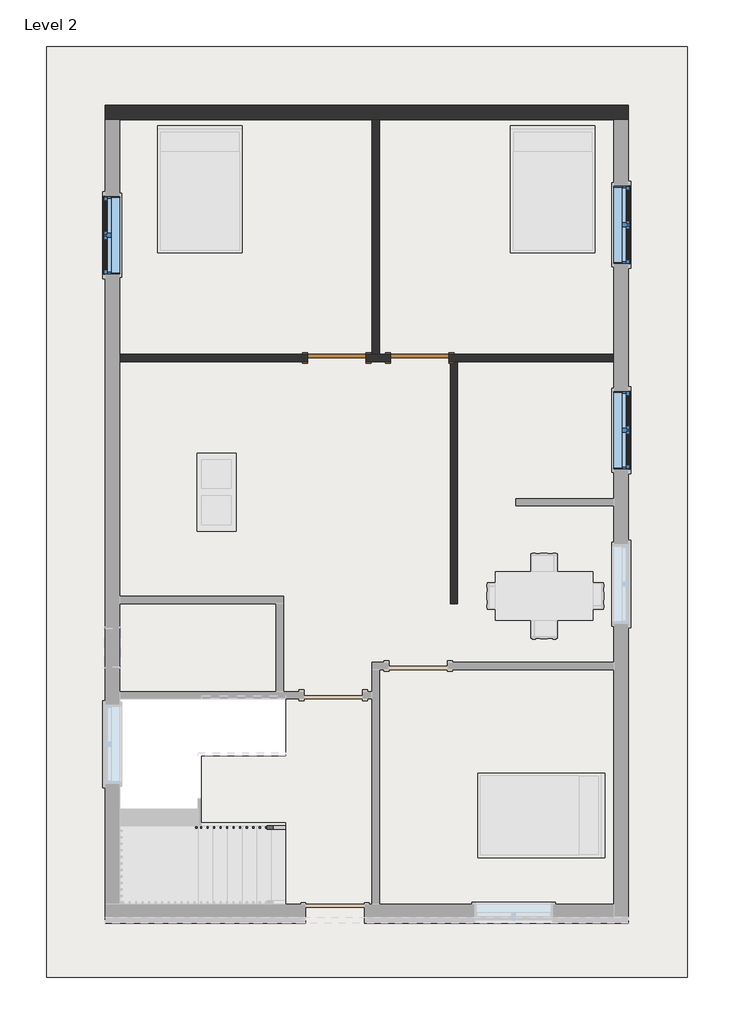
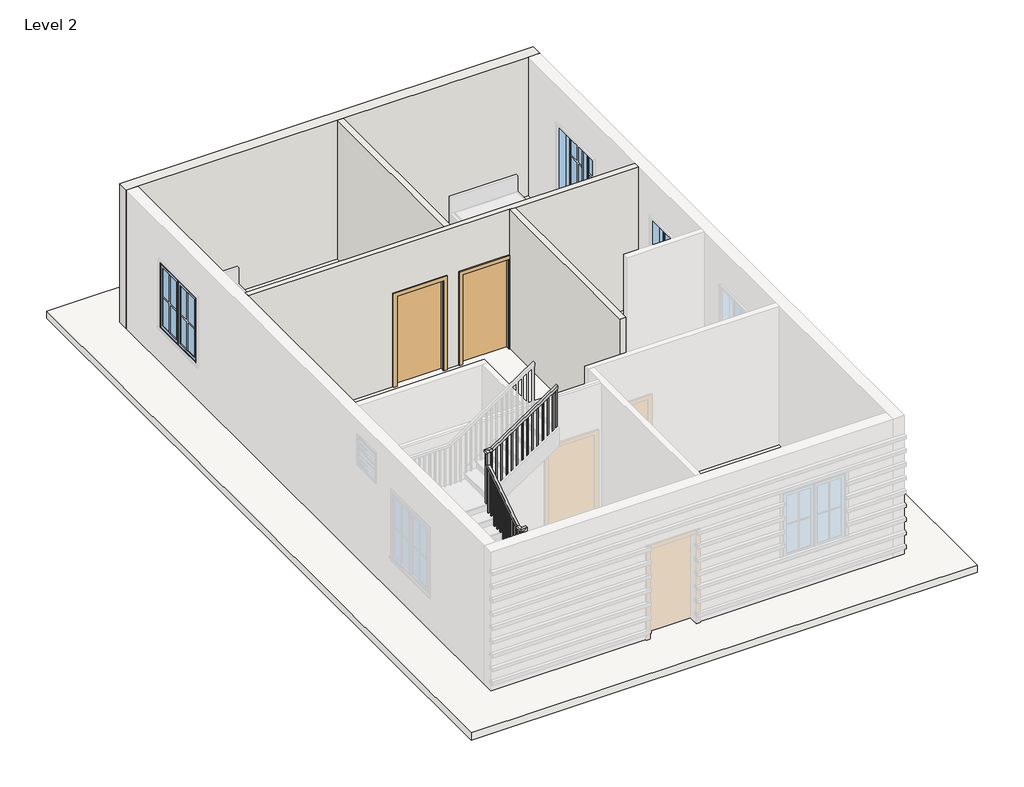
# One storey, part 2 of 3: 4 walls, 3 windows, 2 doors, 1 railing, 1 roof.
"""IFC4 building model written with IfcOpenShell, lengths in millimetres."""

from ifc_helpers import new_model, si_unit, frame, origin, place, context, project, spatial, polyline, outline, extrude, faceted_brep, transform, mapped, element, save
from components import single_flush_door_3_17d80c48, single_flush_door_3_5e62189b, window_casement_double_window_4_576b2d2c

model = new_model("IFC4")

# Units and contexts
model_context = context("Model", 3, world=origin())
ifc_project = project(units=[si_unit("LENGTHUNIT", "METRE", prefix="MILLI")], contexts=[model_context])

# Site, building, storey
site = spatial("IfcSite", under=ifc_project)
building = spatial("IfcBuilding", under=site)
storey = spatial("IfcBuildingStorey", under=building, Name="Level 2", Elevation=3048.0)

# Doors
placement = place(None, origin())
single_flush_door_3_shape = single_flush_door_3_17d80c48(model_context)
element("IfcDoor", 1, ObjectType="Single-Flush : DOOR 3'", at=placement, inside=storey, context=model_context, shape_type="MappedRepresentation", body=[
    mapped(single_flush_door_3_shape, transform((-1721.4617403, 2133.1073441, 3048.0), x_axis=(1.0, 0.0, 0.0), y_axis=(0.0, 1.0, 0.0), z_axis=(0.0, 0.0, 1.0))),
])
single_flush_door_3_2_shape = single_flush_door_3_5e62189b(model_context)
element("IfcDoor", 2, ObjectType="Single-Flush : DOOR 3'", at=placement, inside=storey, context=model_context, shape_type="MappedRepresentation", body=[
    mapped(single_flush_door_3_2_shape, transform((-426.0617403, 2133.1073441, 3048.0), x_axis=(-1.0, 0.0, 0.0), y_axis=(0.0, -1.0, 0.0), z_axis=(0.0, 0.0, 1.0))),
])

# Railing
element("IfcRailing", 3, ObjectType="Handrail - Rectangular", at=placement, inside=storey, context=model_context, shape_type="SolidModel", body=[
    faceted_brep([(-2515.2117403, -5213.8426559, 4114.8), (-2515.2117403, -5213.8426559, 4053.7459984), (-2515.2117403, -5163.0426559, 4053.7459984), (-2515.2117403, -5163.0426559, 4114.8), (-3810.6117403, -5213.8426559, 4978.4), (-3861.4117403, -5213.8426559, 4951.2126651), (-3861.4117403, -5163.0426559, 4951.2126651), (-3810.6117403, -5163.0426559, 4978.4), (-3810.6117403, -5213.8426559, 5232.4), (-3861.4117403, -5213.8426559, 5181.6), (-3861.4117403, -5163.0426559, 5181.6), (-3810.6117403, -5163.0426559, 5232.4), (-3937.6117403, -5213.8426559, 5232.4), (-3937.6117403, -5213.8426559, 5181.6), (-3886.8117403, -5163.0426559, 5181.6), (-3886.8117403, -5163.0426559, 5232.4), (-3937.6117403, -5086.8426559, 5232.4), (-3937.6117403, -5071.4616535, 5181.6), (-3886.8117403, -5071.4616535, 5181.6), (-3886.8117403, -5086.8426559, 5232.4), (-3937.6117403, -4096.2426559, 5892.8), (-3937.6117403, -4045.4426559, 5865.6126651), (-3886.8117403, -4045.4426559, 5865.6126651), (-3886.8117403, -4096.2426559, 5892.8), (-3937.6117403, -4096.2426559, 6146.8), (-3937.6117403, -4045.4426559, 6096.0), (-3886.8117403, -4045.4426559, 6096.0), (-3886.8117403, -4096.2426559, 6146.8), (-3937.6117403, -3969.2426559, 6146.8), (-3937.6117403, -3969.2426559, 6096.0), (-3886.8117403, -4020.0426559, 6096.0), (-3886.8117403, -4020.0426559, 6146.8), (-3810.6117403, -3969.2426559, 6146.8), (-3795.2307379, -3969.2426559, 6096.0), (-3795.2307379, -4020.0426559, 6096.0), (-3810.6117403, -4020.0426559, 6146.8), (-2515.2117403, -3969.2426559, 7010.4), (-2515.2117403, -4020.0426559, 7010.4), (-2515.2117403, -4020.0426559, 6949.3459984), (-2515.2117403, -3969.2426559, 6949.3459984)], [[[0, 1, 2, 3]], [[1, 0, 4, 5]], [[2, 1, 5, 6]], [[3, 2, 6, 7]], [[0, 3, 7, 4]], [[5, 4, 8, 9]], [[6, 5, 9, 10]], [[7, 6, 10, 11]], [[4, 7, 11, 8]], [[9, 8, 12, 13]], [[10, 9, 13, 14]], [[11, 10, 14, 15]], [[8, 11, 15, 12]], [[13, 12, 16, 17]], [[14, 13, 17, 18]], [[15, 14, 18, 19]], [[12, 15, 19, 16]], [[17, 16, 20, 21]], [[18, 17, 21, 22]], [[19, 18, 22, 23]], [[16, 19, 23, 20]], [[21, 20, 24, 25]], [[22, 21, 25, 26]], [[23, 22, 26, 27]], [[20, 23, 27, 24]], [[25, 24, 28, 29]], [[26, 25, 29, 30]], [[27, 26, 30, 31]], [[24, 27, 31, 28]], [[29, 28, 32, 33]], [[30, 29, 33, 34]], [[31, 30, 34, 35]], [[28, 31, 35, 32]], [[36, 37, 38, 39]], [[33, 32, 36, 39]], [[34, 33, 39, 38]], [[35, 34, 38, 37]], [[32, 35, 37, 36]]]),
    extrude(outline(polyline([(6904.8959984, -2581.8867403), (6892.1959984, -2600.9367403), (5943.6, -2600.9367403), (5943.6, -2581.8867403), (6904.8959984, -2581.8867403)])), frame((0.0, -4004.1676559, 0.0), z_axis=(0.0, 1.0, 0.0), x_axis=(0.0, 0.0, 1.0)), (0.0, 0.0, 1.0), 19.05),
    extrude(outline(polyline([(6837.1626651, -2683.4867403), (6824.4626651, -2702.5367403), (5943.6, -2702.5367403), (5943.6, -2683.4867403), (6837.1626651, -2683.4867403)])), frame((0.0, -4004.1676559, 0.0), z_axis=(0.0, 1.0, 0.0), x_axis=(0.0, 0.0, 1.0)), (0.0, 0.0, 1.0), 19.05),
    extrude(outline(polyline([(6769.4293317, -2785.0867403), (6756.7293317, -2804.1367403), (5791.2, -2804.1367403), (5791.2, -2785.0867403), (6769.4293317, -2785.0867403)])), frame((0.0, -4004.1676559, 0.0), z_axis=(0.0, 1.0, 0.0), x_axis=(0.0, 0.0, 1.0)), (0.0, 0.0, 1.0), 19.05),
    extrude(outline(polyline([(6701.6959984, -2886.6867403), (6688.9959984, -2905.7367403), (5791.2, -2905.7367403), (5791.2, -2886.6867403), (6701.6959984, -2886.6867403)])), frame((0.0, -4004.1676559, 0.0), z_axis=(0.0, 1.0, 0.0), x_axis=(0.0, 0.0, 1.0)), (0.0, 0.0, 1.0), 19.05),
    extrude(outline(polyline([(6633.9626651, -2988.2867403), (6621.2626651, -3007.3367403), (5638.8, -3007.3367403), (5638.8, -2988.2867403), (6633.9626651, -2988.2867403)])), frame((0.0, -4004.1676559, 0.0), z_axis=(0.0, 1.0, 0.0), x_axis=(0.0, 0.0, 1.0)), (0.0, 0.0, 1.0), 19.05),
    extrude(outline(polyline([(6566.2293317, -3089.8867403), (6553.5293317, -3108.9367403), (5638.8, -3108.9367403), (5638.8, -3089.8867403), (6566.2293317, -3089.8867403)])), frame((0.0, -4004.1676559, 0.0), z_axis=(0.0, 1.0, 0.0), x_axis=(0.0, 0.0, 1.0)), (0.0, 0.0, 1.0), 19.05),
    extrude(outline(polyline([(6498.4959984, -3191.4867403), (6485.7959984, -3210.5367403), (5638.8, -3210.5367403), (5638.8, -3191.4867403), (6498.4959984, -3191.4867403)])), frame((0.0, -4004.1676559, 0.0), z_axis=(0.0, 1.0, 0.0), x_axis=(0.0, 0.0, 1.0)), (0.0, 0.0, 1.0), 19.05),
    extrude(outline(polyline([(6430.7626651, -3293.0867403), (6418.0626651, -3312.1367403), (5486.4, -3312.1367403), (5486.4, -3293.0867403), (6430.7626651, -3293.0867403)])), frame((0.0, -4004.1676559, 0.0), z_axis=(0.0, 1.0, 0.0), x_axis=(0.0, 0.0, 1.0)), (0.0, 0.0, 1.0), 19.05),
    extrude(outline(polyline([(6363.0293317, -3394.6867403), (6350.3293317, -3413.7367403), (5486.4, -3413.7367403), (5486.4, -3394.6867403), (6363.0293317, -3394.6867403)])), frame((0.0, -4004.1676559, 0.0), z_axis=(0.0, 1.0, 0.0), x_axis=(0.0, 0.0, 1.0)), (0.0, 0.0, 1.0), 19.05),
    extrude(outline(polyline([(6295.2959984, -3496.2867403), (6282.5959984, -3515.3367403), (5334.0, -3515.3367403), (5334.0, -3496.2867403), (6295.2959984, -3496.2867403)])), frame((0.0, -4004.1676559, 0.0), z_axis=(0.0, 1.0, 0.0), x_axis=(0.0, 0.0, 1.0)), (0.0, 0.0, 1.0), 19.05),
    extrude(outline(polyline([(6227.5626651, -3597.8867403), (6214.8626651, -3616.9367403), (5334.0, -3616.9367403), (5334.0, -3597.8867403), (6227.5626651, -3597.8867403)])), frame((0.0, -4004.1676559, 0.0), z_axis=(0.0, 1.0, 0.0), x_axis=(0.0, 0.0, 1.0)), (0.0, 0.0, 1.0), 19.05),
    extrude(outline(polyline([(6159.8293317, -3699.4867403), (6147.1293317, -3718.5367403), (5181.6, -3718.5367403), (5181.6, -3699.4867403), (6159.8293317, -3699.4867403)])), frame((0.0, -4004.1676559, 0.0), z_axis=(0.0, 1.0, 0.0), x_axis=(0.0, 0.0, 1.0)), (0.0, 0.0, 1.0), 19.05),
    extrude(outline(polyline([(6092.0959984, -3801.0867403), (6079.3959984, -3820.1367403), (5181.6, -3820.1367403), (5181.6, -3801.0867403), (6092.0959984, -3801.0867403)])), frame((0.0, -4004.1676559, 0.0), z_axis=(0.0, 1.0, 0.0), x_axis=(0.0, 0.0, 1.0)), (0.0, 0.0, 1.0), 19.05),
    extrude(outline(polyline([(-3902.6867403, -4080.3676559), (-3921.7367403, -4080.3676559), (-3921.7367403, -4061.3176559), (-3902.6867403, -4061.3176559), (-3902.6867403, -4080.3676559)])), frame((0.0, 0.0, 4876.8), z_axis=(0.0, 0.0, 1.0), x_axis=(1.0, 0.0, 0.0)), (0.0, 0.0, 1.0), 1219.2),
    extrude(outline(polyline([(-4181.9676559, 5774.5959984), (-4162.9176559, 5787.2959984), (-4162.9176559, 4876.8), (-4181.9676559, 4876.8), (-4181.9676559, 5774.5959984)])), frame((-3921.7367403, 0.0, 0.0), z_axis=(1.0, 0.0, 0.0), x_axis=(0.0, 1.0, 0.0)), (0.0, 0.0, 1.0), 19.05),
    extrude(outline(polyline([(-4283.5676559, 5706.8626651), (-4264.5176559, 5719.5626651), (-4264.5176559, 4724.4), (-4283.5676559, 4724.4), (-4283.5676559, 5706.8626651)])), frame((-3921.7367403, 0.0, 0.0), z_axis=(1.0, 0.0, 0.0), x_axis=(0.0, 1.0, 0.0)), (0.0, 0.0, 1.0), 19.05),
    extrude(outline(polyline([(-4385.1676559, 5639.1293317), (-4366.1176559, 5651.8293317), (-4366.1176559, 4724.4), (-4385.1676559, 4724.4), (-4385.1676559, 5639.1293317)])), frame((-3921.7367403, 0.0, 0.0), z_axis=(1.0, 0.0, 0.0), x_axis=(0.0, 1.0, 0.0)), (0.0, 0.0, 1.0), 19.05),
    extrude(outline(polyline([(-4486.7676559, 5571.3959984), (-4467.7176559, 5584.0959984), (-4467.7176559, 4724.4), (-4486.7676559, 4724.4), (-4486.7676559, 5571.3959984)])), frame((-3921.7367403, 0.0, 0.0), z_axis=(1.0, 0.0, 0.0), x_axis=(0.0, 1.0, 0.0)), (0.0, 0.0, 1.0), 19.05),
    extrude(outline(polyline([(-4588.3676559, 5503.6626651), (-4569.3176559, 5516.3626651), (-4569.3176559, 4572.0), (-4588.3676559, 4572.0), (-4588.3676559, 5503.6626651)])), frame((-3921.7367403, 0.0, 0.0), z_axis=(1.0, 0.0, 0.0), x_axis=(0.0, 1.0, 0.0)), (0.0, 0.0, 1.0), 19.05),
    extrude(outline(polyline([(-4689.9676559, 5435.9293317), (-4670.9176559, 5448.6293317), (-4670.9176559, 4572.0), (-4689.9676559, 4572.0), (-4689.9676559, 5435.9293317)])), frame((-3921.7367403, 0.0, 0.0), z_axis=(1.0, 0.0, 0.0), x_axis=(0.0, 1.0, 0.0)), (0.0, 0.0, 1.0), 19.05),
    extrude(outline(polyline([(-4791.5676559, 5368.1959984), (-4772.5176559, 5380.8959984), (-4772.5176559, 4419.6), (-4791.5676559, 4419.6), (-4791.5676559, 5368.1959984)])), frame((-3921.7367403, 0.0, 0.0), z_axis=(1.0, 0.0, 0.0), x_axis=(0.0, 1.0, 0.0)), (0.0, 0.0, 1.0), 19.05),
    extrude(outline(polyline([(-4893.1676559, 5300.4626651), (-4874.1176559, 5313.1626651), (-4874.1176559, 4419.6), (-4893.1676559, 4419.6), (-4893.1676559, 5300.4626651)])), frame((-3921.7367403, 0.0, 0.0), z_axis=(1.0, 0.0, 0.0), x_axis=(0.0, 1.0, 0.0)), (0.0, 0.0, 1.0), 19.05),
    extrude(outline(polyline([(-4994.7676559, 5232.7293317), (-4975.7176559, 5245.4293317), (-4975.7176559, 4267.2), (-4994.7676559, 4267.2), (-4994.7676559, 5232.7293317)])), frame((-3921.7367403, 0.0, 0.0), z_axis=(1.0, 0.0, 0.0), x_axis=(0.0, 1.0, 0.0)), (0.0, 0.0, 1.0), 19.05),
    extrude(outline(polyline([(-5096.3676559, 5164.9959984), (-5077.3176559, 5177.6959984), (-5077.3176559, 4267.2), (-5096.3676559, 4267.2), (-5096.3676559, 5164.9959984)])), frame((-3921.7367403, 0.0, 0.0), z_axis=(1.0, 0.0, 0.0), x_axis=(0.0, 1.0, 0.0)), (0.0, 0.0, 1.0), 19.05),
    extrude(outline(polyline([(-3826.4867403, -5178.9176559), (-3826.4867403, -5197.9676559), (-3845.5367403, -5197.9676559), (-3845.5367403, -5178.9176559), (-3826.4867403, -5178.9176559)])), frame((0.0, 0.0, 3962.4), z_axis=(0.0, 0.0, 1.0), x_axis=(1.0, 0.0, 0.0)), (0.0, 0.0, 1.0), 1219.2),
    extrude(outline(polyline([(4860.1959984, -3724.8867403), (4872.8959984, -3743.9367403), (3962.4, -3743.9367403), (3962.4, -3724.8867403), (4860.1959984, -3724.8867403)])), frame((0.0, -5197.9676559, 0.0), z_axis=(0.0, 1.0, 0.0), x_axis=(0.0, 0.0, 1.0)), (0.0, 0.0, 1.0), 19.05),
    extrude(outline(polyline([(4792.4626651, -3623.2867403), (4805.1626651, -3642.3367403), (3810.0, -3642.3367403), (3810.0, -3623.2867403), (4792.4626651, -3623.2867403)])), frame((0.0, -5197.9676559, 0.0), z_axis=(0.0, 1.0, 0.0), x_axis=(0.0, 0.0, 1.0)), (0.0, 0.0, 1.0), 19.05),
    extrude(outline(polyline([(4724.7293317, -3521.6867403), (4737.4293317, -3540.7367403), (3810.0, -3540.7367403), (3810.0, -3521.6867403), (4724.7293317, -3521.6867403)])), frame((0.0, -5197.9676559, 0.0), z_axis=(0.0, 1.0, 0.0), x_axis=(0.0, 0.0, 1.0)), (0.0, 0.0, 1.0), 19.05),
    extrude(outline(polyline([(4656.9959984, -3420.0867403), (4669.6959984, -3439.1367403), (3810.0, -3439.1367403), (3810.0, -3420.0867403), (4656.9959984, -3420.0867403)])), frame((0.0, -5197.9676559, 0.0), z_axis=(0.0, 1.0, 0.0), x_axis=(0.0, 0.0, 1.0)), (0.0, 0.0, 1.0), 19.05),
    extrude(outline(polyline([(4589.2626651, -3318.4867403), (4601.9626651, -3337.5367403), (3657.6, -3337.5367403), (3657.6, -3318.4867403), (4589.2626651, -3318.4867403)])), frame((0.0, -5197.9676559, 0.0), z_axis=(0.0, 1.0, 0.0), x_axis=(0.0, 0.0, 1.0)), (0.0, 0.0, 1.0), 19.05),
    extrude(outline(polyline([(4521.5293317, -3216.8867403), (4534.2293317, -3235.9367403), (3657.6, -3235.9367403), (3657.6, -3216.8867403), (4521.5293317, -3216.8867403)])), frame((0.0, -5197.9676559, 0.0), z_axis=(0.0, 1.0, 0.0), x_axis=(0.0, 0.0, 1.0)), (0.0, 0.0, 1.0), 19.05),
    extrude(outline(polyline([(4453.7959984, -3115.2867403), (4466.4959984, -3134.3367403), (3505.2, -3134.3367403), (3505.2, -3115.2867403), (4453.7959984, -3115.2867403)])), frame((0.0, -5197.9676559, 0.0), z_axis=(0.0, 1.0, 0.0), x_axis=(0.0, 0.0, 1.0)), (0.0, 0.0, 1.0), 19.05),
    extrude(outline(polyline([(4386.0626651, -3013.6867403), (4398.7626651, -3032.7367403), (3505.2, -3032.7367403), (3505.2, -3013.6867403), (4386.0626651, -3013.6867403)])), frame((0.0, -5197.9676559, 0.0), z_axis=(0.0, 1.0, 0.0), x_axis=(0.0, 0.0, 1.0)), (0.0, 0.0, 1.0), 19.05),
    extrude(outline(polyline([(4318.3293317, -2912.0867403), (4331.0293317, -2931.1367403), (3352.8, -2931.1367403), (3352.8, -2912.0867403), (4318.3293317, -2912.0867403)])), frame((0.0, -5197.9676559, 0.0), z_axis=(0.0, 1.0, 0.0), x_axis=(0.0, 0.0, 1.0)), (0.0, 0.0, 1.0), 19.05),
    extrude(outline(polyline([(4250.5959984, -2810.4867403), (4263.2959984, -2829.5367403), (3352.8, -2829.5367403), (3352.8, -2810.4867403), (4250.5959984, -2810.4867403)])), frame((0.0, -5197.9676559, 0.0), z_axis=(0.0, 1.0, 0.0), x_axis=(0.0, 0.0, 1.0)), (0.0, 0.0, 1.0), 19.05),
    extrude(outline(polyline([(4182.8626651, -2708.8867403), (4195.5626651, -2727.9367403), (3200.4, -2727.9367403), (3200.4, -2708.8867403), (4182.8626651, -2708.8867403)])), frame((0.0, -5197.9676559, 0.0), z_axis=(0.0, 1.0, 0.0), x_axis=(0.0, 0.0, 1.0)), (0.0, 0.0, 1.0), 19.05),
    extrude(outline(polyline([(4115.1293317, -2607.2867403), (4127.8293317, -2626.3367403), (3200.4, -2626.3367403), (3200.4, -2607.2867403), (4115.1293317, -2607.2867403)])), frame((0.0, -5197.9676559, 0.0), z_axis=(0.0, 1.0, 0.0), x_axis=(0.0, 0.0, 1.0)), (0.0, 0.0, 1.0), 19.05),
    extrude(outline(polyline([(-3902.6867403, -4004.1676559), (-3921.7367403, -4004.1676559), (-3921.7367403, -3985.1176559), (-3902.6867403, -3985.1176559), (-3902.6867403, -4004.1676559)])), frame((0.0, 0.0, 5029.2), z_axis=(0.0, 0.0, 1.0), x_axis=(1.0, 0.0, 0.0)), (0.0, 0.0, 1.0), 1066.8),
    extrude(outline(polyline([(-3902.6867403, -5178.9176559), (-3902.6867403, -5197.9676559), (-3921.7367403, -5197.9676559), (-3921.7367403, -5178.9176559), (-3902.6867403, -5178.9176559)])), frame((0.0, 0.0, 4114.8), z_axis=(0.0, 0.0, 1.0), x_axis=(1.0, 0.0, 0.0)), (0.0, 0.0, 1.0), 1066.8),
    extrude(outline(polyline([(6949.3459984, -2515.2117403), (6936.6459984, -2534.2617403), (5943.6, -2534.2617403), (5943.6, -2515.2117403), (6949.3459984, -2515.2117403)])), frame((0.0, -4004.1676559, 0.0), z_axis=(0.0, 1.0, 0.0), x_axis=(0.0, 0.0, 1.0)), (0.0, 0.0, 1.0), 19.05),
    extrude(outline(polyline([(4053.7459984, -2515.2117403), (4066.4459984, -2534.2617403), (3200.4, -2534.2617403), (3200.4, -2515.2117403), (4053.7459984, -2515.2117403)])), frame((0.0, -5197.9676559, 0.0), z_axis=(0.0, 1.0, 0.0), x_axis=(0.0, 0.0, 1.0)), (0.0, 0.0, 1.0), 19.05),
])

# Roof
element("IfcRoof", 4, ObjectType="ROOF 6\"", at=placement, inside=storey, context=model_context, shape_type="SweptSolid", body=[
    extrude(outline(polyline([(-6249.0117403, -7525.2426559), (-6249.0117403, 6990.8573441), (3745.8882597, 6990.8573441), (3745.8882597, -7525.2426559), (-6249.0117403, -7525.2426559)]), holes=[polyline([(-5156.8117403, -3131.0426559), (-5156.8117403, -6433.0426559), (-2515.2117403, -6433.0426559), (-2515.2117403, -5112.2426559), (-3836.0117403, -5112.2426559), (-3836.0117403, -4070.8426559), (-2515.2117403, -4070.8426559), (-2515.2117403, -3131.0426559), (-5156.8117403, -3131.0426559)])]), frame((0.0, 0.0, 3048.0), z_axis=(0.0, 0.0, 1.0), x_axis=(1.0, 0.0, 0.0)), (0.0, 0.0, 1.0), 152.4),
])

# Walls
element("IfcWall", 5, ObjectType="ALL 4.5\"", at=placement, inside=storey, context=model_context, shape_type="Brep", body=[
    faceted_brep([(-1264.2617403, 2075.9573441, 3048.0), (-883.2617403, 2075.9573441, 3048.0), (-883.2617403, 2075.9573441, 5080.0), (31.1382597, 2075.9573441, 5080.0), (31.1382597, 2075.9573441, 3048.0), (50.1882597, 2075.9573441, 3048.0), (164.4882597, 2075.9573441, 3048.0), (2602.8882597, 2075.9573441, 3048.0), (2602.8882597, 2075.9573441, 6096.0), (164.4882597, 2075.9573441, 6096.0), (50.1882597, 2075.9573441, 6096.0), (-5106.0117403, 2075.9573441, 6096.0), (-5106.0117403, 2075.9573441, 3048.0), (-2178.6617403, 2075.9573441, 3048.0), (-2178.6617403, 2075.9573441, 5080.0), (-1264.2617403, 2075.9573441, 5080.0), (-883.2617403, 2190.2573441, 5080.0), (-883.2617403, 2190.2573441, 3048.0), (-1054.7117403, 2190.2573441, 3048.0), (-1169.0117403, 2190.2573441, 3048.0), (-1264.2617403, 2190.2573441, 3048.0), (-1264.2617403, 2190.2573441, 5080.0), (-2178.6617403, 2190.2573441, 5080.0), (-2178.6617403, 2190.2573441, 3048.0), (-5106.0117403, 2190.2573441, 3048.0), (-5106.0117403, 2190.2573441, 6096.0), (-1169.0117403, 2190.2573441, 6096.0), (-1054.7117403, 2190.2573441, 6096.0), (2602.8882597, 2190.2573441, 6096.0), (2602.8882597, 2190.2573441, 3048.0), (31.1382597, 2190.2573441, 3048.0), (31.1382597, 2190.2573441, 5080.0)], [[[0, 1, 2, 3, 4, 5, 6, 7, 8, 9, 10, 11, 12, 13, 14, 15]], [[16, 17, 18, 19, 20, 21, 22, 23, 24, 25, 26, 27, 28, 29, 30, 31]], [[13, 12, 24, 23]], [[30, 29, 7, 6, 5, 4]], [[20, 19, 18, 17, 1, 0]], [[8, 7, 29, 28]], [[12, 11, 25, 24]], [[21, 20, 0, 15]], [[22, 21, 15, 14]], [[23, 22, 14, 13]], [[2, 1, 17, 16]], [[3, 2, 16, 31]], [[4, 3, 31, 30]], [[11, 10, 9, 8, 28, 27, 26, 25]]]),
])
element("IfcWall", 6, ObjectType="ALL 4.5\"", at=placement, inside=storey, context=model_context, shape_type="SweptSolid", body=[
    extrude(outline(polyline([(50.1882597, -1695.9426559), (50.1882597, 2075.9573441), (164.4882597, 2075.9573441), (164.4882597, -1695.9426559), (50.1882597, -1695.9426559)])), frame((0.0, 0.0, 3048.0), z_axis=(0.0, 0.0, 1.0), x_axis=(1.0, 0.0, 0.0)), (0.0, 0.0, 1.0), 3048.0),
])
element("IfcWall", 7, ObjectType="ALL 4.5\"", at=placement, inside=storey, context=model_context, shape_type="SweptSolid", body=[
    extrude(outline(polyline([(-1169.0117403, 2190.2573441), (-1169.0117403, 5847.8573441), (-1054.7117403, 5847.8573441), (-1054.7117403, 2190.2573441), (-1169.0117403, 2190.2573441)])), frame((0.0, 0.0, 3048.0), z_axis=(0.0, 0.0, 1.0), x_axis=(1.0, 0.0, 0.0)), (0.0, 0.0, 1.0), 3048.0),
])
element("IfcWall", 8, ObjectType="WALL 9\"", at=placement, inside=storey, context=model_context, shape_type="Brep", body=[
    faceted_brep([(-5334.6117403, 5847.8573441, 3048.0), (-5106.0117403, 5847.8573441, 3048.0), (-1169.0117403, 5847.8573441, 3048.0), (-1054.7117403, 5847.8573441, 3048.0), (2602.8882597, 5847.8573441, 3048.0), (2831.4882597, 5847.8573441, 3048.0), (2831.4882597, 5847.8573441, 6096.0), (2602.8882597, 5847.8573441, 6096.0), (-1054.7117403, 5847.8573441, 6096.0), (-1169.0117403, 5847.8573441, 6096.0), (-5106.0117403, 5847.8573441, 6096.0), (-5334.6117403, 5847.8573441, 6096.0), (-5334.6117403, 6076.4573441, 3048.0), (-5334.6117403, 6076.4573441, 6096.0), (2831.4882597, 6076.4573441, 6096.0), (2831.4882597, 6076.4573441, 3048.0)], [[[0, 1, 2, 3, 4, 5, 6, 7, 8, 9, 10, 11]], [[12, 13, 14, 15]], [[5, 4, 3, 2, 1, 0, 12, 15]], [[6, 5, 15, 14]], [[0, 11, 13, 12]], [[11, 10, 9, 8, 7, 6, 14, 13]]]),
])

# Windows
window_casement_double_window_4_shape = window_casement_double_window_4_576b2d2c(model_context)
element("IfcWindow", 9, ObjectType="Window-Casement-Double : WINDOW 4'", at=placement, inside=storey, context=model_context, shape_type="MappedRepresentation", body=[
    mapped(window_casement_double_window_4_shape, transform((-5220.3117403, 4047.6323441, 3048.0), x_axis=(0.0, 1.0, 0.0), y_axis=(-1.0, 0.0, 0.0), z_axis=(0.0, 0.0, 1.0))),
])
element("IfcWindow", 10, ObjectType="Window-Casement-Double : WINDOW 4'", at=placement, inside=storey, context=model_context, shape_type="MappedRepresentation", body=[
    mapped(window_casement_double_window_4_shape, transform((2717.1882597, 4209.5573441, 3048.0), x_axis=(0.0, -1.0, 0.0), y_axis=(1.0, 0.0, 0.0), z_axis=(0.0, 0.0, 1.0))),
])
element("IfcWindow", 11, ObjectType="Window-Casement-Double : WINDOW 4'", at=placement, inside=storey, context=model_context, shape_type="MappedRepresentation", body=[
    mapped(window_casement_double_window_4_shape, transform((2717.1882597, 1009.1573441, 3048.0), x_axis=(0.0, -1.0, 0.0), y_axis=(1.0, 0.0, 0.0), z_axis=(0.0, 0.0, 1.0))),
])

save(model, "model.ifc")

# Revit data of these elements
# Type "Single-Flush : DOOR 3'"
#   Type Mark = "8"
#   Construction Type Id = "MDOOR"
#   Assembly Code = "C1020"
#   Analytic Construction = "Metal"
#   Thickness = 0' - 2"
#   Heat Transfer Coefficient (U) = 0.651978 BTU/(h·ft²·°F)
#   Height = 6' - 8"
#   Trim Projection Ext = 0' - 1"
#   Trim Projection Int = 0' - 1"
#   Trim Width = 0' - 3"
#   Width = 3' - 0"
#   Define Thermal Properties by = 1
#   Door Material = Door - Panel
#   Frame Material = Door - Frame
#   Visual Light Transmittance = 0
#   Solar Heat Gain Coefficient = 0
#   Function = (empty or 0)
#   Wall Closure = (empty or 0)
# Type "Handrail - Rectangular"
#   Assembly Code = "C2010400"
#   built-in parameter 1008612 = 0.0416667 (stored number, unit not read)
#   built-in parameter 1008611 = 0.0416667 (stored number, unit not read)
#   built-in parameter 1008609 = 0.333333 (stored number, unit not read)
#   built-in parameter 1008604 = 0.166667 (stored number, unit not read)
#   built-in parameter 1008603 = 0.166667 (stored number, unit not read)
#   Railing Height = 3' - 0"
#   built-in parameter 1008630 = 2
#   built-in parameter 1008610 = 2
#   built-in parameter 1008618 = Baluster - Square : 3/4"
# Type "ROOF 6\""
#   Assembly Code = "B1020"
#   Layers, outside or top first: 0' - 6" no material (function 1)
# Type "ALL 4.5\""
#   Assembly Code = "B2010"
#   Layers, outside or top first: 0' - 4 1/2" no material (function 1)
# Type "WALL 9\""
#   Assembly Code = "B2010"
#   Layers, outside or top first: 0' - 9" "Carpet (1)" (function 1)
# Type "Window-Casement-Double : WINDOW 4'"
#   Type Mark = "18"
#   Fire Rating = "0.5h"
#   Assembly Code = "B2020100"
#   Analytic Construction = "Double glazing - domestic"
#   Frame Extension [instance default] = 0' - 0 1/4"
#   Window Inset [instance default] = 0' - 0"
#   Wall Thickness [instance default] = 0' - 6"
#   Interior Wall Closure [instance default] = 0' - 2 1/4"
#   Half Width = 2' - 0"
#   Visual Light Transmittance = 0.81
#   Thermal Resistance (R) = 1.8146 (h·ft²·°F)/BTU
#   Solar Heat Gain Coefficient = 0.76
#   Rough Width = 4' - 0 1/2"
#   Rough Height = 4' - 5 1/2"
#   Height = 4' - 5"
#   Heat Transfer Coefficient (U) = 0.5511 BTU/(h·ft²·°F)
#   Exterior Wall Closure [instance default] = 0' - 1 1/4"
#   Extension Jamb [instance default] = 0' - 2 1/4"
#   Default Sill Height = 3' - 0"
#   Width = 4' - 0"
#   Muntin Visibility = yes
#   Interior Trim Visibility [instance default] = yes
#   Exterior Trim Visibility [instance default] = yes
#   Extension Jamb Visibility [instance default] = yes
#   Interior Trim Material = Wood - Stained
#   Muntin Pattern = Muntin Pattern_2x2 : Muntin Pattern_2x2
#   Interior Trim = Trim-Window-Interior-Flat : Picture Frame
#   Interior Frame Material = Wood - Stained
#   Glass Panel Material = Glass
#   Exterior Trim Material = Clad - White
#   Exterior Trim = Trim-Window-Exterior-Flat : with Sill
#   Exterior Frame Material = Clad - White
#   Wall Closure = (empty or 0)
# Elements 1, 2 (IfcDoor, "Single-Flush : DOOR 3'")
#   Phase Created = New Construction
#   Materials on its faces: "Door - Frame", "Door - Panel"
# Element 3 (IfcRailing, "Handrail - Rectangular")
#   Phase Created = New Construction
#   Materials on its faces: "Clad - White"
# Element 4 (IfcRoof, "ROOF 6\"")
#   built-in parameter 1001705 = 10.5 (stored number, unit not read)
#   built-in parameter 1001710 = 33615
#   Phase Created = New Construction
#   Materials on its faces: "Clad - White", "Default Roof", "Softwood, Lumber"
# Elements 5, 6, 7 (IfcWall, "ALL 4.5\"")
#   Top Offset = 0' - 0"
#   Base Offset = 0' - 0"
#   Unconnected Height = 10' - 0"
#   wall height = 10' - 0"
#   Phase Created = New Construction
#   Base Constraint = Level 2
#   Materials on its faces: "Default Wall"
# Element 8 (IfcWall, "WALL 9\"")
#   Top Offset = 0' - 0"
#   Base Offset = 0' - 0"
#   Unconnected Height = 10' - 0"
#   wall height = 10' - 0"
#   Phase Created = New Construction
#   Base Constraint = Level 2
#   Materials on its faces: "Carpet (1)", "Wood - Stained"
# Element 9 (IfcWindow, "Window-Casement-Double : WINDOW 4'")
#   Mark = "9"
#   Window Inset = 0' - 0"
#   Interior Wall Closure = 0' - 2 1/4"
#   Frame Extension = 0' - 0 1/4"
#   Exterior Wall Closure = 0' - 1 1/4"
#   Interior Trim Visibility = yes
#   Exterior Trim Visibility = yes
#   Phase Created = New Construction
#   Materials on its faces: "Wood - Stained", "Glass", "Clad - White"
# Element 10 (IfcWindow, "Window-Casement-Double : WINDOW 4'")
#   Mark = "10"
#   Window Inset = 0' - 0"
#   Interior Wall Closure = 0' - 2 1/4"
#   Frame Extension = 0' - 0 1/4"
#   Exterior Wall Closure = 0' - 1 1/4"
#   Interior Trim Visibility = yes
#   Exterior Trim Visibility = yes
#   Phase Created = New Construction
#   Materials on its faces: "Wood - Stained", "Glass", "Clad - White"
# Element 11 (IfcWindow, "Window-Casement-Double : WINDOW 4'")
#   Mark = "11"
#   Window Inset = 0' - 0"
#   Interior Wall Closure = 0' - 2 1/4"
#   Frame Extension = 0' - 0 1/4"
#   Exterior Wall Closure = 0' - 1 1/4"
#   Interior Trim Visibility = yes
#   Exterior Trim Visibility = yes
#   Phase Created = New Construction
#   Materials on its faces: "Wood - Stained", "Glass", "Clad - White"
# Materials
#   "Door - Panel": class "Wood", colour RGB 210 159 95, transparency 0, Cost = 0
#   "Door - Frame": colour RGB 118 70 51, transparency 0, Cost = 0
#   "Carpet (1)": class "Carpet", colour RGB 124 80 67, transparency 0, Description = "Interior finish", Cost = 0
#   "Wood - Stained": class "Wood", colour RGB 224 178 126, transparency 0, Cost = 0
#   "Glass": class "Glass", colour RGB 0 128 192, transparency 0.75, Description = "Soda Lime Glass", Cost = 0
#   "Clad - White": class "Wood", colour RGB 242 242 238, transparency 0, Cost = 0
#   "Default Roof": colour RGB 88 101 114, transparency 0, Cost = 0
#   "Softwood, Lumber": class "Wood", colour RGB 223 192 134, transparency 0, Description = "Pinus Echinata", Cost = 0
#   "Default Wall": colour RGB 128 128 128, transparency 0, Cost = 0
